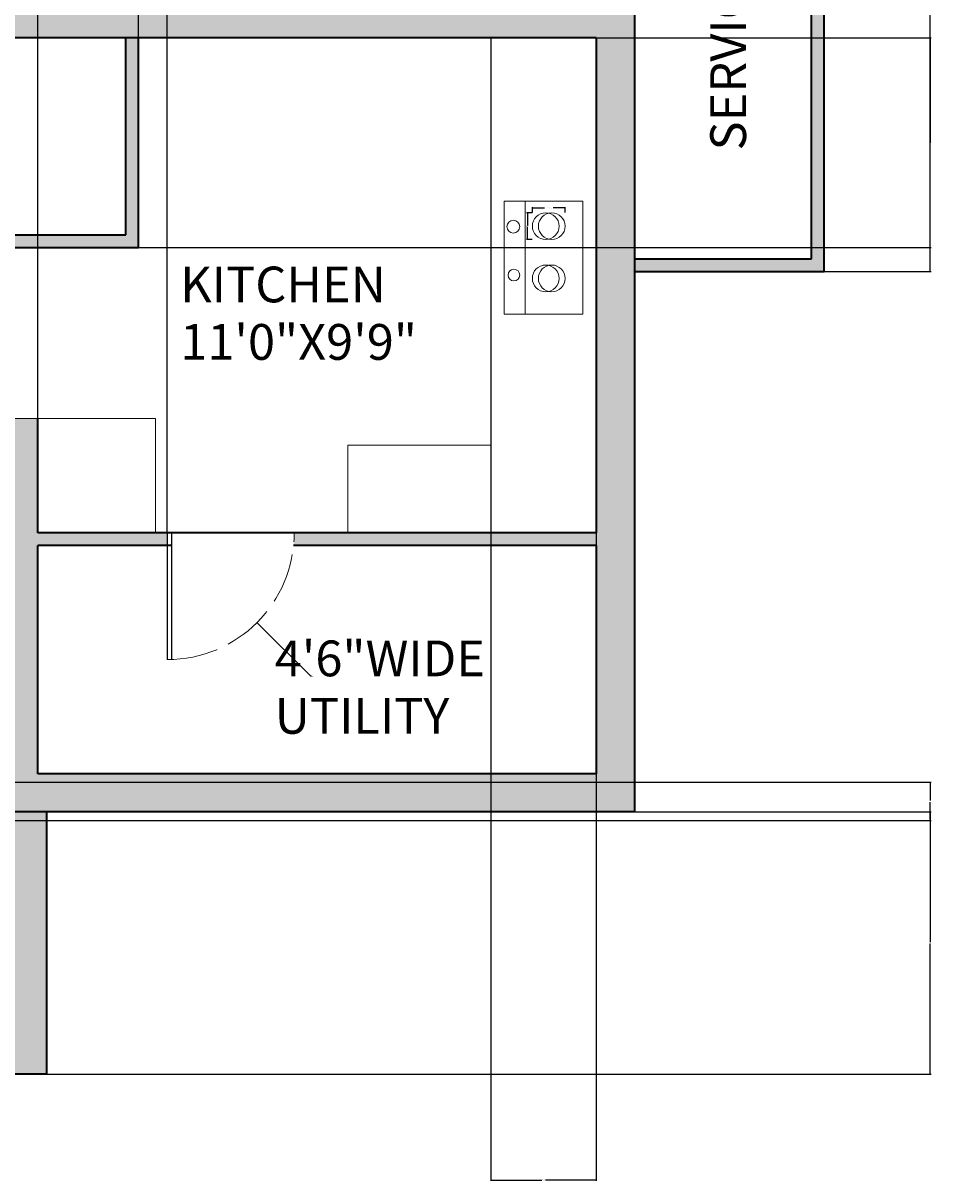
# Model space of a CAD drawing. Units: inches. Extents: x -12 to 539, y -477 to 51.
# Tile 4 of 6: x 325 to 539, y -477 to -203. Entities that reach past the tile are written whole.
import ezdxf

# ---------------------------------------------------------------- set-up
doc = ezdxf.new("R2010")
doc.units = ezdxf.units.IN
doc.header["$MEASUREMENT"] = 0
doc.linetypes.add('ACAD_ISO02W100', pattern=[15, 12, -3])
for name, color, linetype, lineweight in [('A-ANNO-DIMS', 2, 'Continuous', 18), ('A-AREA-IDEN', 7, 'Continuous', 18), ('A-DOOR', 4, 'Continuous', 25), ('A-DOOR-SWNG', 4, 'ACAD_ISO02W100', 13), ('A-EQPM', 8, 'Continuous', 18), ('A-FLOR-CASE', 9, 'Continuous', 18), ('A-WALL', 7, 'Continuous', 35)]:
    doc.layers.add(name, color=color, linetype=linetype, lineweight=lineweight)
doc.layers.add('A-WALL-PATT', color=252, linetype='Continuous', lineweight=13, true_color=0x939598)
doc.styles.get("Standard").update_dxf_attribs({"font": 'arial.ttf'})
doc.dimstyles.get("Standard").update_dxf_attribs({"dimtxt": 0.18, "dimasz": 0.18, "dimexe": 0.18, "dimexo": 0.0625, "dimgap": 0.09, "dimtad": 0, "dimtih": 1, "dimtoh": 1, "dimdec": 0, "dimzin": 0, "dimdsep": 46, "dimlunit": 3, "dimtxsty": 'Standard', "dimcen": 0.09, "dimadec": 0, "dimazin": 0, "dimtfac": 1, "dimtdec": 0, "dimtofl": 0, "dimtmove": 0, "dimatfit": 3, "dimfxl": 1, "dimtolj": 1, "dimtzin": 0, "dimarcsym": 0})

# ---------------------------------------------------------------- blocks, each defined once
blk = doc.blocks.new('COOKTOP-BURNER')
for centre in [(3.16, 3.16), (4.59, 3.16)]:
    blk.add_circle(centre, 3.16)
blk = doc.blocks.new('*D27')
at = {"layer": 'A-ANNO-DIMS', "color": 0, "lineweight": -2, "transparency": 16777216}
for p, q in [((444.98, -248.28), (444.98, -247)), ((445.16, -247.18), (447.83, -247.18)), ((452.54, -247.18), (449.87, -247.18)), ((452.72, -248.28), (452.72, -247))]:
    blk.add_line(p, q, dxfattribs=at)
at = {"layer": 'A-ANNO-DIMS', "color": 0, "transparency": 16777216}
for points in [[(445.16, -247.15), (445.16, -247.21), (444.98, -247.18)], [(452.54, -247.15), (452.54, -247.21), (452.72, -247.18)]]:
    blk.add_solid(points, dxfattribs=at)
at = {"layer": 'Defpoints', "color": 0, "transparency": 16777216}
for p in [(444.98, -248.35), (452.72, -247.18), (452.72, -248.35)]:
    blk.add_point(p, dxfattribs=at)
at = {"layer": 'A-ANNO-DIMS', "color": 0, "transparency": 16777216, "insert": (448.85, -247.18), "char_height": 0.18, "attachment_point": 5}
blk.add_mtext('\\A1;BURNER 8 TYP.', dxfattribs=at)
blk = doc.blocks.new('*D28')
at = {"layer": 'A-ANNO-DIMS', "color": 0, "lineweight": -2, "transparency": 16777216}
for p, q in [((444.91, -248.35), (443.63, -248.35)), ((443.81, -248.53), (443.81, -251.32)), ((443.81, -254.48), (443.81, -251.68)), ((444.91, -254.66), (443.63, -254.66))]:
    blk.add_line(p, q, dxfattribs=at)
at = {"layer": 'A-ANNO-DIMS', "color": 0, "transparency": 16777216}
for points in [[(443.78, -248.53), (443.84, -248.53), (443.81, -248.35)], [(443.78, -254.48), (443.84, -254.48), (443.81, -254.66)]]:
    blk.add_solid(points, dxfattribs=at)
at = {"layer": 'Defpoints', "color": 0, "transparency": 16777216}
for p in [(443.81, -248.35), (444.98, -248.35), (444.98, -254.66)]:
    blk.add_point(p, dxfattribs=at)
at = {"layer": 'A-ANNO-DIMS', "color": 0, "transparency": 16777216, "insert": (443.81, -251.5), "char_height": 0.18, "attachment_point": 5}
blk.add_mtext('\\A1;6 TYP.', dxfattribs=at)
blk = doc.blocks.new('*D40')
at = {"layer": 'A-ANNO-DIMS', "color": 0, "lineweight": -2, "transparency": 16777216}
for p, q in [((514.05, -124.99), (539.23, -124.99)), ((539.05, -125.17), (539.05, -193.41)), ((539.05, -262.02), (539.05, -193.78)), ((514.05, -262.2), (539.23, -262.2))]:
    blk.add_line(p, q, dxfattribs=at)
at = {"layer": 'A-ANNO-DIMS', "color": 0, "transparency": 16777216}
for points in [[(539.02, -125.17), (539.08, -125.17), (539.05, -124.99)], [(539.02, -262.02), (539.08, -262.02), (539.05, -262.2)]]:
    blk.add_solid(points, dxfattribs=at)
at = {"layer": 'Defpoints', "color": 0, "transparency": 16777216}
for p in [(513.99, -124.99), (513.99, -262.2), (539.05, -262.2)]:
    blk.add_point(p, dxfattribs=at)
at = {"layer": 'A-ANNO-DIMS', "color": 0, "transparency": 16777216, "insert": (539.05, -193.6), "char_height": 0.18, "attachment_point": 5}
blk.add_mtext('\\A1;137.22', dxfattribs=at)
blk = doc.blocks.new('*D44')
at = {"layer": 'A-ANNO-DIMS', "color": 0, "lineweight": -2, "transparency": 16777216}
for p, q in [((330.17, -389.99), (539.23, -389.99)), ((539.05, -390.17), (539.05, -420.81)), ((539.05, -451.81), (539.05, -421.17)), ((330.17, -451.99), (539.23, -451.99))]:
    blk.add_line(p, q, dxfattribs=at)
at = {"layer": 'A-ANNO-DIMS', "color": 0, "transparency": 16777216}
for points in [[(539.02, -390.17), (539.08, -390.17), (539.05, -389.99)], [(539.02, -451.81), (539.08, -451.81), (539.05, -451.99)]]:
    blk.add_solid(points, dxfattribs=at)
at = {"layer": 'Defpoints', "color": 0, "transparency": 16777216}
for p in [(330.1, -389.99), (539.05, -389.99), (330.1, -451.99)]:
    blk.add_point(p, dxfattribs=at)
at = {"layer": 'A-ANNO-DIMS', "color": 0, "transparency": 16777216, "insert": (539.05, -420.99), "char_height": 0.18, "attachment_point": 5}
blk.add_mtext('\\A1;62', dxfattribs=at)
blk = doc.blocks.new('*D45')
at = {"layer": 'A-ANNO-DIMS', "color": 0, "lineweight": -2, "transparency": 16777216}
for p, q in [((22.17, -382.99), (539.23, -382.99)), ((539.05, -383.17), (539.05, -387.31)), ((539.05, -391.81), (539.05, -387.67)), ((13.17, -391.99), (539.23, -391.99))]:
    blk.add_line(p, q, dxfattribs=at)
at = {"layer": 'A-ANNO-DIMS', "color": 0, "transparency": 16777216}
for points in [[(539.02, -383.17), (539.08, -383.17), (539.05, -382.99)], [(539.02, -391.81), (539.08, -391.81), (539.05, -391.99)]]:
    blk.add_solid(points, dxfattribs=at)
at = {"layer": 'Defpoints', "color": 0, "transparency": 16777216}
for p in [(22.1, -382.99), (539.05, -382.99), (13.1, -391.99)]:
    blk.add_point(p, dxfattribs=at)
at = {"layer": 'A-ANNO-DIMS', "color": 0, "transparency": 16777216, "insert": (539.05, -387.49), "char_height": 0.18, "attachment_point": 5}
blk.add_mtext('\\A1;9', dxfattribs=at)
blk = doc.blocks.new('*D51')
at = {"layer": 'A-ANNO-DIMS', "color": 0, "lineweight": -2, "transparency": 16777216}
for p, q in [((328.1, -323.93), (328.1, 51.25)), ((328.28, 51.07), (342.93, 51.07)), ((358.5, 51.07), (343.85, 51.07)), ((358.68, -323.93), (358.68, 51.25))]:
    blk.add_line(p, q, dxfattribs=at)
at = {"layer": 'A-ANNO-DIMS', "color": 0, "transparency": 16777216}
for points in [[(328.28, 51.1), (328.28, 51.04), (328.1, 51.07)], [(358.5, 51.1), (358.5, 51.04), (358.68, 51.07)]]:
    blk.add_solid(points, dxfattribs=at)
at = {"layer": 'Defpoints', "color": 0, "transparency": 16777216}
for p in [(358.68, 51.07), (328.1, -323.99), (358.68, -323.99)]:
    blk.add_point(p, dxfattribs=at)
at = {"layer": 'A-ANNO-DIMS', "color": 0, "transparency": 16777216, "insert": (343.39, 51.07), "char_height": 0.18, "attachment_point": 5}
blk.add_mtext('\\A1;30.574', dxfattribs=at)
blk = doc.blocks.new('*D52')
at = {"layer": 'A-ANNO-DIMS', "color": 0, "lineweight": -2, "transparency": 16777216}
for p, q in [((435.2, -207.05), (435.2, -477.23)), ((460.1, -207.05), (460.1, -477.23)), ((435.38, -477.05), (447.19, -477.05)), ((459.92, -477.05), (448.12, -477.05))]:
    blk.add_line(p, q, dxfattribs=at)
at = {"layer": 'A-ANNO-DIMS', "color": 0, "transparency": 16777216}
for points in [[(435.38, -477.02), (435.38, -477.08), (435.2, -477.05)], [(459.92, -477.02), (459.92, -477.08), (460.1, -477.05)]]:
    blk.add_solid(points, dxfattribs=at)
at = {"layer": 'Defpoints', "color": 0, "transparency": 16777216}
for p in [(435.2, -206.99), (460.1, -206.99), (460.1, -477.05)]:
    blk.add_point(p, dxfattribs=at)
at = {"layer": 'A-ANNO-DIMS', "color": 0, "transparency": 16777216, "insert": (447.65, -477.05), "char_height": 0.18, "attachment_point": 5}
blk.add_mtext('\\A1;24.903', dxfattribs=at)
blk = doc.blocks.new('*D55')
at = {"layer": 'A-ANNO-DIMS', "color": 0, "lineweight": -2, "transparency": 16777216}
for p, q in [((351.95, -206.99), (539.23, -206.99)), ((539.05, -207.17), (539.05, -231.59)), ((539.05, -256.37), (539.05, -231.95)), ((351.95, -256.55), (539.23, -256.55))]:
    blk.add_line(p, q, dxfattribs=at)
at = {"layer": 'A-ANNO-DIMS', "color": 0, "transparency": 16777216}
for points in [[(539.02, -207.17), (539.08, -207.17), (539.05, -206.99)], [(539.02, -256.37), (539.08, -256.37), (539.05, -256.55)]]:
    blk.add_solid(points, dxfattribs=at)
at = {"layer": 'Defpoints', "color": 0, "transparency": 16777216}
for p in [(351.88, -206.99), (351.88, -256.55), (539.05, -256.55)]:
    blk.add_point(p, dxfattribs=at)
at = {"layer": 'A-ANNO-DIMS', "color": 0, "transparency": 16777216, "insert": (539.05, -231.77), "char_height": 0.18, "attachment_point": 5}
blk.add_mtext('\\A1;49.56', dxfattribs=at)
blk = doc.blocks.new('*D56')
at = {"layer": 'A-ANNO-DIMS', "color": 0, "lineweight": -2, "transparency": 16777216}
for p, q in [((321.1, -256.48), (321.1, 51.25)), ((321.28, 51.07), (336.1, 51.07)), ((351.7, 51.07), (336.89, 51.07)), ((351.88, -256.48), (351.88, 51.25))]:
    blk.add_line(p, q, dxfattribs=at)
at = {"layer": 'A-ANNO-DIMS', "color": 0, "transparency": 16777216}
for points in [[(321.28, 51.1), (321.28, 51.04), (321.1, 51.07)], [(351.7, 51.1), (351.7, 51.04), (351.88, 51.07)]]:
    blk.add_solid(points, dxfattribs=at)
at = {"layer": 'Defpoints', "color": 0, "transparency": 16777216}
for p in [(351.88, 51.07), (321.1, -256.55), (351.88, -256.55)]:
    blk.add_point(p, dxfattribs=at)
at = {"layer": 'A-ANNO-DIMS', "color": 0, "transparency": 16777216, "insert": (336.49, 51.07), "char_height": 0.18, "attachment_point": 5}
blk.add_mtext('\\A1;30.78', dxfattribs=at)
blk = doc.blocks.new('*D67')
at = {"layer": 'A-ANNO-DIMS', "color": 0, "lineweight": -2, "transparency": 16777216}
for p, q in [((358.59, -323.99), (358.77, -323.99)), ((358.68, -324.08), (358.68, -323.9)), ((392.62, -357.93), (380.02, -345.33)), ((392.8, -357.93), (392.62, -357.93))]:
    blk.add_line(p, q, dxfattribs=at)
at = {"layer": 'A-ANNO-DIMS', "color": 0, "transparency": 16777216}
blk.add_solid([(380.04, -345.31), (380, -345.35), (379.89, -345.2)], dxfattribs=at)
at = {"layer": 'Defpoints', "color": 0, "transparency": 16777216}
for p in [(358.68, -323.99), (379.89, -345.2)]:
    blk.add_point(p, dxfattribs=at)
at = {"layer": 'A-ANNO-DIMS', "color": 0, "transparency": 16777216, "insert": (393.1, -357.93), "char_height": 0.18, "attachment_point": 5}
blk.add_mtext('\\A1;R30', dxfattribs=at)

msp = doc.modelspace()

# ---------------------------------------------------------------- hatches: boundary and pattern name
at = {"layer": 'A-WALL-PATT'}
h = msp.add_hatch(color=256, dxfattribs=at)
h.dxf.hatch_style = 1
h.paths.add_polyline_path([(267.143, 26.0124), (13.1031, 26.0124), (13.1031, -391.9876), (177.1031, -391.9876), (177.1031, -346.9876), (307.7315, -346.9876), (321.1031, -346.9876), (321.1031, -389.9876), (469.1031, -389.9876), (469.1031, 26.0124), (302.7142, 26.0124), (302.7142, 17.0124), (321.1031, 17.0124), (321.1031, -131.577, -0.04877504), (328.1031, -132.2621), (328.1031, 17.0124), (460.1031, 17.0124), (460.1031, -124.9876), (382.1031, -124.9876), (379.1031, -124.9876), (379.1031, -131.5624), (382.1031, -131.5624), (382.1031, -127.9876), (460.1031, -127.9876), (460.1031, -153.7747), (460.1031, -199.9876), (382.1031, -199.9876), (382.1031, -167.7132), (379.1031, -167.7132), (379.1031, -199.9876), (328.1031, -199.9876), (328.1031, -167.7132), (321.1031, -167.7132), (321.1031, -206.9876), (460.1031, -206.9876), (460.1031, -323.9876), (388.677, -323.9876, -0.02504709), (388.5266, -326.9876), (460.1031, -326.9876), (460.1031, -380.9876), (328.1031, -380.9876), (328.1031, -326.9876), (358.677, -326.9876), (358.677, -323.9876), (328.1031, -323.9876), (328.1031, -296.9562), (321.1031, -296.9562), (321.1031, -339.9876), (307.7315, -339.9876), (177.1031, -339.9876), (177.1031, -250.9876), (244.0259, -250.9876), (244.0259, -243.9876), (163.7315, -243.9876), (163.7315, -250.9876), (170.1031, -250.9876), (170.1031, -382.9876), (22.1031, -382.9876), (22.1031, -250.9876), (41.3871, -250.9876, -0.06888376), (40.8612, -243.9876), (22.1031, -243.9876), (22.1031, -183.9876), (118.1031, -183.9876), (118.1031, -243.9876), (71.6031, -243.9876), (71.6031, -250.9876), (128.4772, -250.9876, -0.04900189), (127.7315, -243.9876), (121.1031, -243.9876), (121.1031, -183.9876), (121.1031, -120.9876), (118.1031, -120.9876), (118.1031, -180.9876), (22.1031, -180.9876), (22.1031, -120.9876), (49.0045, -120.9876, -0.07000725), (46.9084, -111.9876), (46.1728, -111.9876), (22.1031, -111.9876), (22.1031, 17.0124), (170.1031, 17.0124), (170.1031, -120.9876), (177.1031, -120.9876), (177.1031, 17.0124), (268.2584, 17.0124, -0.0639977)])
h.paths.add_polyline_path([(513.9866, -124.9876), (469.1031, -124.9876), (469.1031, -127.9876), (510.9866, -127.9876), (510.9866, -259.2045), (469.1031, -259.2045), (469.1031, -262.2045), (513.9866, -262.2045)])
h.paths.add_polyline_path([(351.8833, -206.9876), (348.8833, -206.9876), (348.8833, -253.547), (328.1031, -253.547), (321.1031, -253.547), (321.1031, -256.547), (328.1031, -256.547), (351.8833, -256.547)], flags=17)
h.paths.add_polyline_path([(330.1031, -389.9876), (321.1031, -389.9876), (321.1031, -442.9876), (177.1031, -442.9876), (177.1031, -391.9876), (168.1031, -391.9876), (168.1031, -451.9876), (330.1031, -451.9876)])
h.paths.add_polyline_path([(414.1504, -177.6962), (465.5248, -177.6962), (465.5248, -164.7437), (414.1504, -164.7437)], flags=25)

# ---------------------------------------------------------------- linework, layer by layer
at = {"layer": 'A-DOOR'}
for p, q in [((358.677, -323.9876), (358.677, -353.9876)), ((359.677, -323.9876), (359.677, -353.9876))]:
    msp.add_line(p, q, dxfattribs=at)
at = {"layer": 'A-DOOR-SWNG'}
msp.add_line((358.677, -323.9876), (388.677, -323.9876), dxfattribs=at)
msp.add_arc((358.677, -323.9876), 30, 270, 0, dxfattribs=at)
at = {"layer": 'A-EQPM'}
msp.add_line((443.2752, -245.6087), (443.2752, -272.2805), dxfattribs=at)
msp.add_lwpolyline([(438.3474, -245.6087), (456.899, -245.6087), (456.899, -272.2805), (438.3474, -272.2805)], close=True, dxfattribs=at)
for centre, radius in [((440.4779, -251.5975), 1.5201), ((440.6162, -263.0671), 1.3819)]:
    msp.add_circle(centre, radius, dxfattribs=at)
at = {"layer": 'A-FLOR-CASE'}
for p, q in [((435.2, -303.2745), (435.2, -206.9876)), ((321.1031, -296.9562), (355.8953, -296.9562)), ((355.8953, -296.9562), (355.8953, -323.9876)), ((401.3909, -323.9876), (401.3909, -303.2745)), ((401.3909, -303.2745), (435.2, -303.2745))]:
    msp.add_line(p, q, dxfattribs=at)
at = {"layer": 'A-WALL'}
for p, q in [((469.1031, 26.0124), (469.1031, -389.9876)), ((513.9866, -262.2045), (513.9866, -124.9876)), ((510.9866, -259.2045), (510.9866, -127.9876)), ((460.1031, -206.9876), (321.1031, -206.9876)), ((348.8833, -253.547), (348.8833, -206.9876)), ((351.8833, -256.547), (351.8833, -206.9876)), ((460.1031, -206.9876), (460.1031, -323.9876)), ((321.1031, -253.547), (328.1031, -253.547)), ((328.1031, -253.547), (348.8833, -253.547)), ((321.1031, -256.547), (328.1031, -256.547)), ((328.1031, -256.547), (351.8833, -256.547)), ((469.1031, -259.2045), (510.9866, -259.2045)), ((469.1031, -262.2045), (513.9866, -262.2045)), ((328.1031, -323.9876), (328.1031, -296.9562)), ((460.1031, -323.9876), (328.1031, -323.9876)), ((328.1031, -380.9876), (328.1031, -326.9876)), ((359.677, -326.9876), (328.1031, -326.9876)), ((460.1031, -326.9876), (388.5266, -326.9876)), ((460.1031, -326.9876), (460.1031, -380.9876)), ((469.1031, -326.9876), (469.1031, -380.9876)), ((460.1031, -380.9876), (328.1031, -380.9876)), ((469.1031, -389.9876), (321.1031, -389.9876)), ((330.1031, -389.9876), (330.1031, -451.9876)), ((330.1031, -451.9876), (168.1031, -451.9876))]:
    msp.add_line(p, q, dxfattribs=at)

# ---------------------------------------------------------------- block references
at = {"layer": 'A-EQPM'}
for p in [(444.976, -254.657), (444.976, -267.0057)]:
    msp.add_blockref('COOKTOP-BURNER', p, dxfattribs=at)

# ---------------------------------------------------------------- texts
at = {"layer": 'A-AREA-IDEN'}
msp.add_text('SERVICE LEDGE', height=8.456178, rotation=90, dxfattribs=at).set_placement((495.4985, -233.5965))
for s, p in [('KITCHEN', (361.733, -269.5054)), ('11\'0"X9\'9"', (361.733, -283.0895)), ('4\'6"WIDE', (384.0682, -357.9233)), ('UTILITY', (384.0682, -371.5074))]:
    msp.add_text(s, height=8.45618, dxfattribs=at).set_placement(p)

# ---------------------------------------------------------------- dimensions: what is measured, and where the dimension line sits
at = {"layer": 'A-ANNO-DIMS'}
for base, p1, p2, override, picture, middle in [((351.8833, 51.0724), (321.1031, -256.547), (351.8833, -256.547), {"dimdec": 2, "dimlfac": 1, "dimrnd": 0, "dimzin": 0, "dimdsep": 46, "dimlunit": 2}, '*D56', (336.4932, 51.0724)), ((358.677, 51.0724), (328.1031, -323.9876), (358.677, -323.9876), {"dimdec": 3, "dimlfac": 1, "dimrnd": 0, "dimzin": 0, "dimdsep": 46, "dimlunit": 2}, '*D51', (343.39, 51.0724)), ((460.1031, -477.0476), (435.2, -206.9876), (460.1031, -206.9876), {"dimdec": 3, "dimlfac": 1, "dimrnd": 0, "dimzin": 0, "dimdsep": 46, "dimlunit": 2}, '*D52', (447.6515, -477.0476))]:
    dim = msp.add_linear_dim(base=base, p1=p1, p2=p2, dimstyle='Standard', override=override, dxfattribs=at)
    dim.commit()
    dim.dimension.update_dxf_attribs({"geometry": picture, "text_midpoint": middle})
for base, p1, p2, override, picture, middle in [((539.0466, -262.2045), (513.9866, -124.9876), (513.9866, -262.2045), {"dimdec": 2, "dimlfac": 1, "dimrnd": 0, "dimzin": 0, "dimdsep": 46, "dimlunit": 2}, '*D40', (539.0466, -193.596)), ((539.0466, -256.547), (351.8833, -206.9876), (351.8833, -256.547), {"dimdec": 2, "dimlfac": 1, "dimrnd": 0, "dimzin": 0, "dimdsep": 46, "dimlunit": 2}, '*D55', (539.0466, -231.7673)), ((539.0466, -382.9876), (13.1031, -391.9876), (22.1031, -382.9876), {"dimdec": 0, "dimlfac": 1, "dimrnd": 0, "dimzin": 0, "dimdsep": 46, "dimlunit": 2}, '*D45', (539.0466, -387.4876)), ((539.0466, -389.9876), (330.1031, -451.9876), (330.1031, -389.9876), {"dimdec": 0, "dimlfac": 1, "dimrnd": 0, "dimzin": 0, "dimdsep": 46, "dimlunit": 2}, '*D44', (539.0466, -420.9876))]:
    dim = msp.add_linear_dim(base=base, p1=p1, p2=p2, angle=90, dimstyle='Standard', override=override, dxfattribs=at)
    dim.commit()
    dim.dimension.update_dxf_attribs({"geometry": picture, "text_midpoint": middle})
dim = msp.add_linear_dim(base=(443.8144, -248.3456), p1=(444.9764, -254.6572), p2=(444.9764, -248.3456), angle=90, text='<> TYP.', dimstyle='Standard', override={"dimdec": 0, "dimlfac": 1, "dimrnd": 0, "dimzin": 0, "dimdsep": 46, "dimlunit": 2}, dxfattribs=at)
dim.commit()
dim.dimension.update_dxf_attribs({"geometry": '*D28', "text_midpoint": (443.8144, -251.5014)})
dim = msp.add_linear_dim(base=(452.723, -247.1836), p1=(444.9764, -248.3456), p2=(452.723, -248.3456), text='BURNER <> TYP.', dimstyle='Standard', override={"dimdec": 0, "dimlfac": 1, "dimrnd": 0, "dimzin": 0, "dimdsep": 46, "dimlunit": 2}, dxfattribs=at)
dim.commit()
dim.dimension.update_dxf_attribs({"geometry": '*D27', "text_midpoint": (448.8497, -247.1836)})
dim = msp.add_radius_dim(center=(358.677, -323.9876), mpoint=(379.89, -345.201), dimstyle='Standard', override={"dimdec": 0, "dimlfac": 1, "dimrnd": 0, "dimzin": 0, "dimdsep": 46, "dimlunit": 2}, dxfattribs=at)
dim.commit()
dim.dimension.update_dxf_attribs({"geometry": '*D67', "text_midpoint": (393.1025, -357.9291), "dimtype": 164})

doc.saveas('drawing.dxf')
